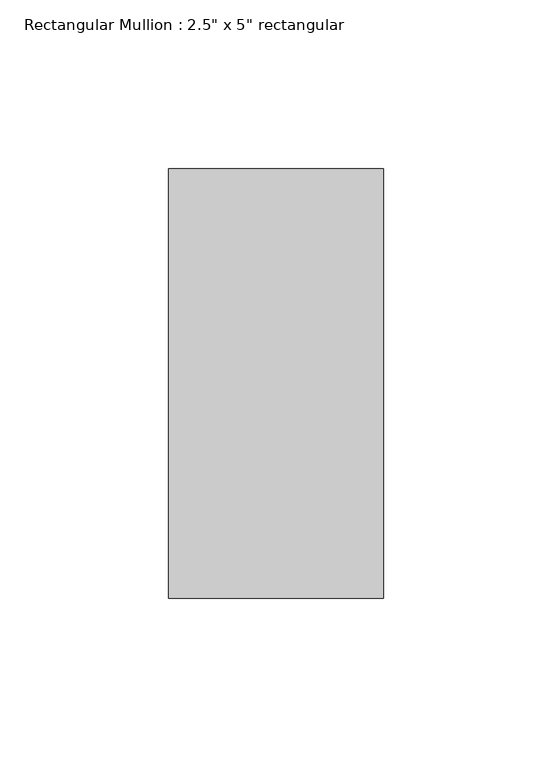
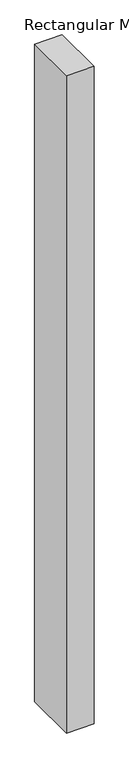
"""IFC4 building model written with IfcOpenShell, lengths in millimetres: member geometry."""

from ifc_helpers import new_model, si_unit, frame, origin, place, context, project, spatial, polyline, outline, extrude, source, transform, mapped, element, save


def member_87fdabbb(model_context):
    return source(origin(), model_context, "Body", "SweptSolid", [
        extrude(outline(polyline([(0.0, 63.5), (0.0, -63.5), (-63.5, -63.5), (-63.5, 63.5), (0.0, 63.5)])), frame((0.0, 0.0, -1603.3915419), z_axis=(0.0, 0.0, 1.0), x_axis=(1.0, 0.0, 0.0)), (0.0, 0.0, 1.0), 1603.3915419),
    ])


if __name__ == "__main__":
    model = new_model("IFC4")
    model_context = context("Model", 3, world=origin())
    ifc_project = project(units=[si_unit("LENGTHUNIT", "METRE", prefix="MILLI")], contexts=[model_context])
    site = spatial("IfcSite", under=ifc_project)
    building = spatial("IfcBuilding", under=site)
    placement = place(None, origin())
    member_shape = member_87fdabbb(model_context)
    element("IfcMember", 1, ObjectType="Rectangular Mullion : 2.5\" x 5\" rectangular", at=placement, inside=building, context=model_context, shape_type="MappedRepresentation", body=[
        mapped(member_shape, transform((0.0, 0.0, 0.0), x_axis=(1.0, 0.0, 0.0), y_axis=(0.0, 1.0, 0.0), z_axis=(0.0, 0.0, 1.0))),
    ])
    save(model, "model.ifc")

# Revit data of these elements
# Type "Rectangular Mullion : 2.5\" x 5\" rectangular"
#   built-in parameter 1007304 = 0.416667 (stored number, unit not read)
#   built-in parameter 1007301 = 0.104167 (stored number, unit not read)
#   built-in parameter 1007300 = 0.104167 (stored number, unit not read)
# Element 1 (IfcMember, "Rectangular Mullion : 2.5\" x 5\" rectangular")
#   Materials on its faces: "Aluminum"
# Materials
#   "Aluminum": class "Metal", colour RGB 247 247 247, transparency 0, Description = "Aluminum 6061", Cost = 0
